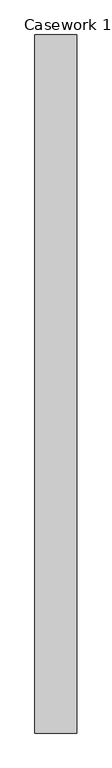
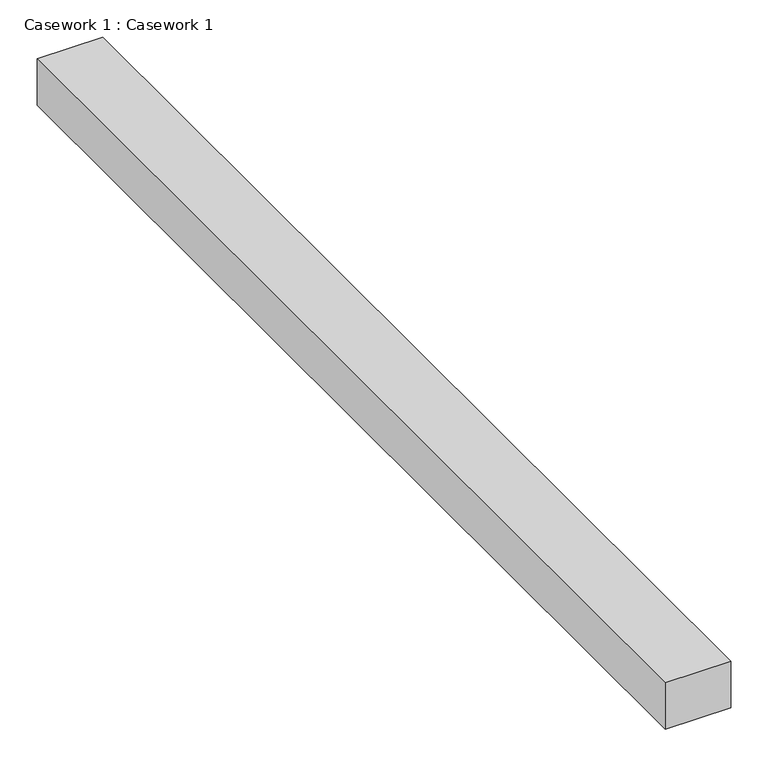
"""IFC4 building model written with IfcOpenShell, lengths in millimetres: furniture geometry, Casework 1 : Casework 1."""

from ifc_helpers import new_model, si_unit, frame, origin, place, context, project, spatial, polyline, outline, extrude, source, transform, mapped, element, save


def casework_1_casework_1_f574b021(model_context):
    return source(origin(), model_context, "Body", "SweptSolid", [
        extrude(outline(polyline([(9662.5559589, 14787.9496924), (9662.5559589, 13098.8496924), (9560.9559589, 13098.8496924), (9560.9559589, 14787.9496924), (9662.5559589, 14787.9496924)])), frame((0.0, 0.0, 3581.4), z_axis=(0.0, 0.0, 1.0), x_axis=(1.0, 0.0, 0.0)), (0.0, 0.0, 1.0), 76.2),
    ])


if __name__ == "__main__":
    model = new_model("IFC4")
    model_context = context("Model", 3, world=origin())
    ifc_project = project(units=[si_unit("LENGTHUNIT", "METRE", prefix="MILLI")], contexts=[model_context])
    site = spatial("IfcSite", under=ifc_project)
    building = spatial("IfcBuilding", under=site)
    placement = place(None, origin())
    casework_1_casework_1_shape = casework_1_casework_1_f574b021(model_context)
    element("IfcFurniture", 1, ObjectType="Casework 1 : Casework 1", at=placement, inside=building, context=model_context, shape_type="MappedRepresentation", body=[
        mapped(casework_1_casework_1_shape, transform((0.0, 0.0, 0.0), x_axis=(1.0, 0.0, 0.0), y_axis=(0.0, 1.0, 0.0), z_axis=(0.0, 0.0, 1.0))),
    ])
    save(model, "model.ifc")

# Revit data of these elements
# Element 1 (IfcFurniture, "Casework 1 : Casework 1")
#   Materials on its faces: "Clad - White"
# Materials
#   "Clad - White": class "Wood", colour RGB 242 242 238, transparency 0, Cost = 0
